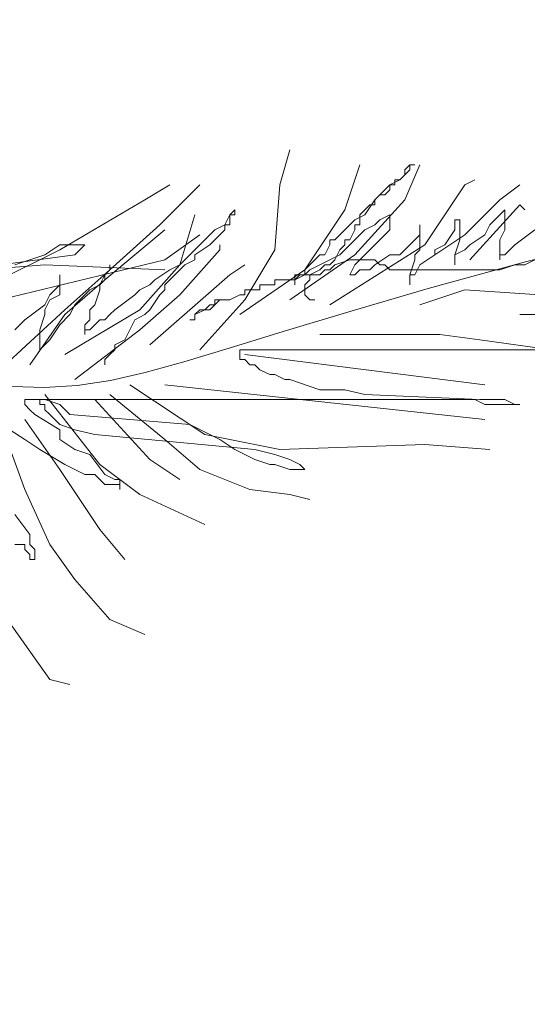
# Model space of a CAD drawing. Units: millimetres. Extents: x 595116 to 630915, y 909473 to 920225.
# Tile 85 of 134: x 629724.653 to 629727.558, y 919270.048 to 919275.684. Entities that reach past the tile are written whole.
import ezdxf

# ---------------------------------------------------------------- set-up
doc = ezdxf.new("R2010")
doc.units = ezdxf.units.MM
doc.layers.add('Dimension', color=3, linetype='Continuous', lineweight=18)
doc.layers.add('L-PLNT', color=85, linetype='Continuous', lineweight=13)
doc.styles.get("Standard").update_dxf_attribs({"font": 'arial.ttf'})
doc.dimstyles.new('ISO-25', dxfattribs={"dimtxt": 9, "dimasz": 6, "dimexe": 1.25, "dimexo": 0.625, "dimtad": 1, "dimlunit": 4, "dimtxsty": 'Standard', "dimcen": 2.5, "dimadec": 0, "dimazin": 0, "dimtfac": 1, "dimtmove": 0, "dimatfit": 3, "dimfxl": 1, "dimarcsym": 0})

# ---------------------------------------------------------------- blocks, each defined once
blk = doc.blocks.new('A$C4FB75ABC')
for p, q in [((4.2249, 2.058), (4.2402, 2.1114)), ((4.324, 2.0199), (4.3469, 2.0885)), ((4.4156, 2.0809), (4.4232, 2.0885)), ((4.4156, 2.0352), (4.4384, 2.0885)), ((4.4232, 2.0885), (4.4308, 2.0885)), ((4.4308, 2.0885), (4.4232, 2.0885)), ((4.4232, 2.0885), (4.4232, 2.0809)), ((4.4079, 2.0657), (4.4156, 2.0733)), ((4.4156, 2.0733), (4.4079, 2.0657)), ((4.4156, 2.0733), (4.4156, 2.0809)), ((4.4232, 2.0809), (4.4156, 2.0733)), ((4.019, 2.0352), (4.0571, 2.058)), ((4.0419, 1.9971), (4.1029, 2.058)), ((4.2173, 1.9589), (4.2249, 2.058)), ((4.3927, 2.058), (4.3851, 2.0504)), ((4.4079, 2.0657), (4.3927, 2.058)), ((4.3927, 2.0504), (4.3927, 2.058)), ((4.3927, 2.058), (4.4003, 2.058)), ((4.4003, 2.058), (4.4003, 2.0657)), ((4.4003, 2.0657), (4.4079, 2.0657)), ((4.4461, 1.9666), (4.5071, 2.058)), ((4.5071, 2.058), (4.5223, 2.0657)), ((4.5605, 2.0352), (4.591, 2.058)), ((4.3698, 2.0352), (4.3774, 2.0428)), ((4.3774, 2.0428), (4.3698, 2.0352)), ((4.3851, 2.0504), (4.3774, 2.0428)), ((4.3774, 2.0428), (4.3851, 2.0428)), ((4.3851, 2.0428), (4.3927, 2.0504)), ((3.8894, 1.9589), (4.019, 2.0352)), ((4.3393, 1.9513), (4.4156, 2.0352)), ((4.3469, 2.0123), (4.3622, 2.0275)), ((4.3698, 2.0352), (4.3546, 2.0123)), ((4.3622, 2.0275), (4.3698, 2.0275)), ((4.3698, 2.0275), (4.3698, 2.0352)), ((4.5071, 1.9818), (4.5605, 2.0352)), ((4.5147, 1.9437), (4.591, 2.0275)), ((4.591, 2.0275), (4.5986, 2.0199)), ((4.0724, 1.9361), (4.0953, 2.0123)), ((4.1486, 2.0123), (4.141, 1.9971)), ((4.1563, 2.0199), (4.1486, 2.0123)), ((4.1486, 1.9971), (4.1486, 2.0123)), ((4.1486, 2.0123), (4.1563, 2.0123)), ((4.1563, 2.0123), (4.1563, 2.0199)), ((4.263, 1.9285), (4.324, 2.0199)), ((4.3546, 2.0123), (4.3393, 2.0047)), ((4.3469, 1.9971), (4.3469, 2.0123)), ((4.3774, 2.0047), (4.3927, 2.0123)), ((4.3927, 2.0123), (4.3927, 1.9894)), ((4.5528, 2.0047), (4.5605, 2.0123)), ((4.5605, 2.0123), (4.5681, 2.0199)), ((4.5681, 2.0199), (4.5681, 1.9894)), ((4.3393, 2.0047), (4.3317, 1.9971)), ((4.3698, 1.9971), (4.3774, 2.0047)), ((4.4918, 1.9894), (4.4918, 2.0047)), ((4.4918, 2.0047), (4.4995, 2.0047)), ((4.4995, 2.0047), (4.4995, 1.9742)), ((4.5452, 1.9971), (4.5528, 2.0047)), ((3.958, 1.9132), (4.0495, 1.9894)), ((3.9656, 1.9285), (4.0419, 1.9971)), ((4.1258, 1.9894), (4.1181, 1.9818)), ((4.141, 1.9971), (4.1258, 1.9894)), ((4.1334, 1.9818), (4.141, 1.9894)), ((4.141, 1.9894), (4.141, 1.9971)), ((4.141, 1.9971), (4.1486, 1.9971)), ((4.3317, 1.9971), (4.3164, 1.9818)), ((4.3317, 1.9742), (4.3393, 1.9894)), ((4.3393, 1.9894), (4.3393, 1.9971)), ((4.3393, 1.9971), (4.3469, 1.9971)), ((4.3469, 1.9818), (4.3546, 1.9894)), ((4.3546, 1.9894), (4.3698, 1.9971)), ((4.3927, 1.9894), (4.3851, 1.9818)), ((4.4384, 1.9818), (4.4384, 1.9971)), ((4.4384, 1.9971), (4.4384, 1.9589)), ((4.4766, 1.9666), (4.4918, 1.9894)), ((4.5376, 1.9818), (4.5452, 1.9971)), ((4.5681, 1.9894), (4.5605, 1.9742)), ((4.5833, 1.9666), (4.6138, 1.9894)), ((4.7725, 1.9851), (4.5975, 1.9398)), ((4.0495, 1.9437), (4.1029, 1.9818)), ((4.1181, 1.9818), (4.1029, 1.9666)), ((4.1181, 1.9666), (4.1334, 1.9818)), ((4.3088, 1.9742), (4.3012, 1.9742)), ((4.3012, 1.9742), (4.3012, 1.9666)), ((4.3164, 1.9818), (4.3088, 1.9742)), ((4.3164, 1.9513), (4.3469, 1.9818)), ((4.324, 1.9666), (4.324, 1.9742)), ((4.324, 1.9742), (4.3317, 1.9742)), ((4.3851, 1.9818), (4.3698, 1.9666)), ((4.4156, 1.9589), (4.4308, 1.9742)), ((4.4308, 1.9742), (4.4384, 1.9818)), ((4.4384, 1.9361), (4.5071, 1.9818)), ((4.4995, 1.9742), (4.4918, 1.9513)), ((4.5147, 1.9666), (4.5376, 1.9818)), ((4.5605, 1.9742), (4.5605, 1.9437)), ((3.7521, 1.8903), (3.8894, 1.9589)), ((3.8894, 1.9666), (3.8665, 1.9513)), ((3.9275, 1.9666), (3.8894, 1.9666)), ((3.9122, 1.9513), (3.9199, 1.9589)), ((3.9199, 1.9589), (3.9275, 1.9666)), ((4.0724, 1.8903), (4.1334, 1.9589)), ((4.1029, 1.9666), (4.08, 1.9437)), ((4.0953, 1.9513), (4.1181, 1.9666)), ((4.1334, 1.9589), (4.1334, 1.9666)), ((4.1715, 1.8827), (4.2173, 1.9589)), ((4.3012, 1.9666), (4.2935, 1.9513)), ((4.3012, 1.8751), (4.4461, 1.9666)), ((4.3088, 1.9437), (4.3164, 1.9589)), ((4.3164, 1.9589), (4.324, 1.9666)), ((4.3622, 1.9589), (4.3469, 1.9437)), ((4.3698, 1.9666), (4.3622, 1.9589)), ((4.4079, 1.9513), (4.4156, 1.9589)), ((4.4384, 1.9589), (4.4308, 1.9513)), ((4.4613, 1.9589), (4.4766, 1.9666)), ((4.4613, 1.9513), (4.4613, 1.9589)), ((4.4918, 1.9513), (4.5071, 1.9589)), ((4.5071, 1.9589), (4.5147, 1.9666)), ((4.5681, 1.9513), (4.5757, 1.9589)), ((4.5757, 1.9589), (4.5833, 1.9666)), ((3.7445, 1.9285), (3.9122, 1.9513)), ((3.7978, 1.8827), (4.0495, 1.9437)), ((3.8665, 1.9513), (3.8207, 1.9361)), ((4.08, 1.9437), (4.0724, 1.9361)), ((4.08, 1.9361), (4.0953, 1.9437)), ((4.0953, 1.9437), (4.0953, 1.9513)), ((4.2402, 1.8827), (4.3393, 1.9513)), ((4.2859, 1.9513), (4.2707, 1.9361)), ((4.2707, 1.9285), (4.3012, 1.9437)), ((4.2935, 1.9513), (4.2859, 1.9513)), ((4.3012, 1.9437), (4.3164, 1.9513)), ((4.3012, 1.9361), (4.3088, 1.9437)), ((4.3317, 1.9437), (4.3088, 1.9361)), ((4.3698, 1.9437), (4.3317, 1.9437)), ((4.3469, 1.9437), (4.3393, 1.9361)), ((4.3698, 1.9361), (4.3927, 1.9513)), ((4.3774, 1.9361), (4.3698, 1.9437)), ((4.3927, 1.9513), (4.4079, 1.9513)), ((4.4308, 1.9437), (4.4232, 1.9208)), ((4.4308, 1.9513), (4.4308, 1.9437)), ((4.4384, 1.9361), (4.4613, 1.9513)), ((4.5975, 1.9398), (4.4513, 1.8996)), ((4.4918, 1.9513), (4.4918, 1.9361)), ((4.4918, 1.9361), (4.4918, 1.9513)), ((4.5605, 1.9513), (4.5681, 1.9513)), ((4.5605, 1.9437), (4.5605, 1.9513)), ((4.6138, 1.9437), (4.5986, 1.9361)), ((3.5843, 1.9132), (3.8665, 1.9361)), ((3.8665, 1.9361), (4.0495, 1.9285)), ((3.897, 1.8675), (3.9656, 1.9285)), ((3.958, 1.9208), (3.9656, 1.9285)), ((3.9656, 1.9285), (3.958, 1.9208)), ((3.9656, 1.9285), (3.9656, 1.9361)), ((3.9656, 1.9361), (3.9656, 1.9285)), ((4.0114, 1.8675), (4.0724, 1.9361)), ((4.0571, 1.9285), (4.0343, 1.9132)), ((4.0724, 1.9361), (4.0571, 1.9285)), ((4.0571, 1.9132), (4.0724, 1.9285)), ((4.0724, 1.9285), (4.08, 1.9361)), ((4.1486, 1.9208), (4.1715, 1.9361)), ((4.1639, 1.8599), (4.263, 1.9285)), ((4.2707, 1.9361), (4.263, 1.9285)), ((4.263, 1.9285), (4.263, 1.9208)), ((4.263, 1.9208), (4.2707, 1.9285)), ((4.2707, 1.9208), (4.2859, 1.9285)), ((4.2859, 1.9285), (4.2935, 1.9361)), ((4.2935, 1.9285), (4.2859, 1.9208)), ((4.2935, 1.9361), (4.3012, 1.9361)), ((4.3012, 1.9285), (4.2935, 1.9285)), ((4.3088, 1.9361), (4.3012, 1.9285)), ((4.3393, 1.9361), (4.3317, 1.9208)), ((4.3393, 1.9208), (4.3469, 1.9285)), ((4.3469, 1.9285), (4.3622, 1.9285)), ((4.3622, 1.9285), (4.3698, 1.9361)), ((4.3851, 1.9361), (4.3774, 1.9361)), ((4.3927, 1.9285), (4.3851, 1.9361)), ((4.5605, 1.9285), (4.3927, 1.9285)), ((4.4308, 1.9208), (4.4384, 1.9361)), ((4.5833, 1.9361), (4.5605, 1.9285)), ((4.5986, 1.9361), (4.5833, 1.9361)), ((3.8894, 1.8903), (3.8894, 1.9208)), ((3.8894, 1.9208), (3.8894, 1.9056)), ((3.897, 1.8599), (3.958, 1.9132)), ((3.958, 1.9208), (3.9504, 1.9056)), ((3.9504, 1.9056), (3.958, 1.9132)), ((3.958, 1.9132), (3.958, 1.9208)), ((4.0266, 1.8141), (4.1486, 1.9208)), ((4.0343, 1.9132), (4.0266, 1.9056)), ((4.0495, 1.9056), (4.0571, 1.9132)), ((4.2478, 1.9132), (4.2173, 1.9132)), ((4.2173, 1.9132), (4.2173, 1.9056)), ((4.2554, 1.9208), (4.2478, 1.9132)), ((4.2478, 1.9056), (4.2478, 1.9208)), ((4.2478, 1.9208), (4.263, 1.9208)), ((4.263, 1.9208), (4.2478, 1.9132)), ((4.2478, 1.9132), (4.2478, 1.9056)), ((4.263, 1.9208), (4.2554, 1.9208)), ((4.2859, 1.9208), (4.263, 1.9208)), ((4.263, 1.9056), (4.2707, 1.9132)), ((4.2707, 1.9132), (4.2707, 1.9208)), ((4.3317, 1.9208), (4.3393, 1.9208)), ((4.4232, 1.9208), (4.4232, 1.9056)), ((4.4232, 1.9056), (4.4232, 1.9208)), ((4.4232, 1.9208), (4.4308, 1.9208)), ((3.8894, 1.9056), (3.8741, 1.8903)), ((3.9351, 1.898), (3.9122, 1.8751)), ((3.9504, 1.9056), (3.9351, 1.898)), ((3.9427, 1.8751), (3.9504, 1.898)), ((3.9504, 1.898), (3.9504, 1.9056)), ((4.0114, 1.898), (4.0037, 1.8903)), ((4.0266, 1.9056), (4.0114, 1.898)), ((4.0419, 1.8903), (4.0495, 1.898)), ((4.0495, 1.898), (4.0495, 1.9056)), ((4.1944, 1.898), (4.1715, 1.898)), ((4.1715, 1.898), (4.1715, 1.8903)), ((4.2173, 1.9056), (4.1944, 1.9056)), ((4.1944, 1.9056), (4.1944, 1.898)), ((4.263, 1.8903), (4.263, 1.9056)), ((4.4513, 1.8996), (4.3302, 1.8644)), ((4.4384, 1.8751), (4.5071, 1.898)), ((4.5071, 1.898), (4.6215, 1.8903)), ((3.8741, 1.8903), (3.8665, 1.8751)), ((3.8665, 1.8675), (3.8741, 1.8827)), ((3.8741, 1.8827), (3.8894, 1.8903)), ((4.0037, 1.8903), (3.9732, 1.8675)), ((4.0114, 1.837), (4.0724, 1.8903)), ((4.0266, 1.8675), (4.0419, 1.8903)), ((4.1029, 1.8065), (4.1715, 1.8827)), ((4.1334, 1.8827), (4.1258, 1.8751)), ((4.1258, 1.8751), (4.1258, 1.8827)), ((4.1258, 1.8827), (4.1334, 1.8827)), ((4.1486, 1.8827), (4.1334, 1.8827)), ((4.1639, 1.8903), (4.1486, 1.8827)), ((4.1715, 1.8903), (4.1639, 1.8903)), ((4.2707, 1.8827), (4.263, 1.8903)), ((4.2783, 1.8827), (4.2707, 1.8827)), ((3.7978, 1.776), (3.897, 1.8675)), ((3.8665, 1.8751), (3.836, 1.8522)), ((3.8665, 1.8599), (3.8665, 1.8675)), ((3.897, 1.7989), (4.0114, 1.8675)), ((3.9122, 1.8751), (3.9046, 1.8599)), ((3.9351, 1.8675), (3.9427, 1.8751)), ((3.9351, 1.8522), (3.9351, 1.8675)), ((3.9732, 1.8675), (3.9656, 1.8599)), ((4.019, 1.8599), (4.0266, 1.8675)), ((4.1029, 1.8675), (4.0953, 1.8599)), ((4.0953, 1.8599), (4.1105, 1.8675)), ((4.1105, 1.8675), (4.1029, 1.8675)), ((4.1181, 1.8751), (4.1105, 1.8675)), ((4.1105, 1.8675), (4.1181, 1.8675)), ((4.1258, 1.8751), (4.1181, 1.8751)), ((4.1181, 1.8675), (4.1258, 1.8751)), ((4.3302, 1.8644), (4.2303, 1.8341)), ((3.836, 1.8522), (3.8207, 1.837)), ((3.8436, 1.7836), (3.897, 1.8599)), ((3.8589, 1.837), (3.8665, 1.8599)), ((3.9046, 1.8599), (3.8894, 1.8446)), ((3.9275, 1.8446), (3.9351, 1.8522)), ((3.9504, 1.8522), (3.9427, 1.8446)), ((3.958, 1.8522), (3.9504, 1.8522)), ((3.9656, 1.8599), (3.958, 1.8522)), ((3.9885, 1.8217), (4.0037, 1.8522)), ((4.0037, 1.8522), (4.019, 1.8599)), ((4.0953, 1.8522), (4.0876, 1.8522)), ((4.0876, 1.8522), (4.0953, 1.8522)), ((4.0953, 1.8599), (4.0953, 1.8522)), ((4.0953, 1.8522), (4.0953, 1.8599)), ((4.6062, 1.8599), (4.591, 1.8599)), ((4.591, 1.8599), (4.652, 1.8599)), ((3.8589, 1.8065), (3.8589, 1.837)), ((3.8894, 1.8446), (3.8741, 1.8217)), ((3.9122, 1.7608), (4.0114, 1.837)), ((3.9275, 1.8294), (3.9275, 1.8446)), ((3.9351, 1.837), (3.9275, 1.837)), ((3.9275, 1.837), (3.9275, 1.8294)), ((3.9427, 1.8446), (3.9351, 1.837)), ((4.2303, 1.8341), (4.1477, 1.8087)), ((3.8741, 1.8217), (3.8665, 1.8141)), ((3.9732, 1.8141), (3.9885, 1.8217)), ((4.2859, 1.8294), (4.4689, 1.8294)), ((4.4689, 1.8294), (4.53, 1.8217)), ((4.53, 1.8217), (4.6367, 1.8065)), ((3.8665, 1.8141), (3.8589, 1.8065)), ((3.9656, 1.7989), (3.9732, 1.8065)), ((3.9732, 1.8065), (3.9732, 1.8141)), ((4.1477, 1.8087), (4.0788, 1.7878)), ((4.1639, 1.7913), (4.1639, 1.8065)), ((4.1639, 1.8065), (5.0333, 1.8065)), ((3.958, 1.7913), (3.9656, 1.7989)), ((3.958, 1.7836), (3.958, 1.7913)), ((4.0788, 1.7878), (4.0197, 1.7715)), ((4.1715, 1.7913), (4.1639, 1.7913)), ((4.1715, 1.7989), (4.5376, 1.7531)), ((4.1792, 1.7836), (4.1715, 1.7913)), ((4.1868, 1.7836), (4.1792, 1.7836)), ((4.1944, 1.776), (4.1868, 1.7836)), ((4.2097, 1.7684), (4.1944, 1.776)), ((3.9666, 1.7597), (3.916, 1.7521)), ((4.0197, 1.7715), (3.9666, 1.7597)), ((4.2173, 1.7684), (4.2097, 1.7684)), ((4.2325, 1.7608), (4.2173, 1.7684)), ((4.2402, 1.7608), (4.2325, 1.7608)), ((4.2859, 1.7455), (4.2402, 1.7608)), ((3.8664, 1.749), (3.8165, 1.7504)), ((3.916, 1.7521), (3.8664, 1.749)), ((3.9961, 1.7531), (4.1105, 1.6769)), ((4.0495, 1.7531), (4.5376, 1.6998)), ((4.324, 1.7455), (4.2859, 1.7455)), ((4.3546, 1.7379), (4.324, 1.7455)), ((3.836, 1.7227), (3.836, 1.7303)), ((3.836, 1.7303), (3.8665, 1.7303)), ((3.8589, 1.7227), (3.8589, 1.7303)), ((3.8589, 1.7303), (4.5223, 1.7303)), ((3.8665, 1.7379), (3.9504, 1.6312)), ((3.8665, 1.7303), (3.8894, 1.7227)), ((3.9427, 1.7303), (4.0266, 1.6388)), ((3.9656, 1.7379), (4.0495, 1.6693)), ((4.53, 1.7303), (4.3546, 1.7379)), ((4.5223, 1.7303), (4.5376, 1.7227)), ((4.5681, 1.7303), (4.53, 1.7303)), ((4.5833, 1.7227), (4.5681, 1.7303)), ((3.8436, 1.715), (3.836, 1.7227)), ((3.8512, 1.7074), (3.8436, 1.715)), ((3.8665, 1.7227), (3.8589, 1.7227)), ((3.8665, 1.715), (3.8665, 1.7227)), ((3.8741, 1.7074), (3.8665, 1.715)), ((3.8894, 1.7227), (3.9046, 1.7074)), ((4.5376, 1.7227), (4.591, 1.7227)), ((4.591, 1.7227), (4.5833, 1.7227)), ((3.836, 1.6998), (3.8894, 1.6236)), ((3.8894, 1.6845), (3.8512, 1.7074)), ((3.8894, 1.6922), (3.8741, 1.7074)), ((3.9046, 1.7074), (4.0876, 1.6922)), ((3.8131, 1.6845), (3.836, 1.6693)), ((3.9122, 1.6845), (3.8894, 1.6922)), ((3.8894, 1.6693), (3.8894, 1.6845)), ((3.9427, 1.6769), (3.9122, 1.6845)), ((4.0876, 1.6922), (4.1181, 1.6769)), ((3.8055, 1.6769), (3.836, 1.5931)), ((3.836, 1.6693), (3.8589, 1.6541)), ((3.9122, 1.6541), (3.8894, 1.6693)), ((4.1868, 1.6541), (3.9427, 1.6769)), ((4.0495, 1.6693), (4.1029, 1.6236)), ((4.1105, 1.6769), (4.2249, 1.6541)), ((4.1181, 1.6769), (4.1334, 1.6693)), ((4.1334, 1.6693), (4.1563, 1.6541)), ((3.8589, 1.6541), (3.897, 1.6312)), ((3.9351, 1.6464), (3.9122, 1.6541)), ((4.1563, 1.6541), (4.1868, 1.6388)), ((4.2173, 1.6464), (4.1868, 1.6541)), ((4.2249, 1.6541), (4.4461, 1.6617)), ((4.4461, 1.6617), (4.5452, 1.6541)), ((3.958, 1.6159), (3.9351, 1.6464)), ((4.0266, 1.6388), (4.0724, 1.6083)), ((4.1868, 1.6388), (4.2097, 1.6312)), ((4.2402, 1.6388), (4.2173, 1.6464)), ((4.2554, 1.6312), (4.2402, 1.6388)), ((3.8894, 1.6236), (3.9504, 1.5321)), ((3.897, 1.6312), (3.9275, 1.6159)), ((3.9504, 1.6312), (4.0114, 1.5855)), ((4.1029, 1.6236), (4.1792, 1.5931)), ((4.2097, 1.6312), (4.2173, 1.6312)), ((4.2173, 1.6312), (4.2402, 1.6236)), ((4.2402, 1.6236), (4.263, 1.6236)), ((4.263, 1.6236), (4.2554, 1.6312)), ((3.9275, 1.6159), (3.9427, 1.6159)), ((3.9427, 1.6159), (3.958, 1.6007)), ((3.9732, 1.6083), (3.958, 1.6159)), ((3.9809, 1.6083), (3.9732, 1.6083)), ((3.9809, 1.5931), (3.9809, 1.6083)), ((3.836, 1.5931), (3.8741, 1.5092)), ((3.958, 1.6007), (3.9809, 1.6007)), ((3.9809, 1.6007), (3.9809, 1.5931)), ((4.1792, 1.5931), (4.2402, 1.5855)), ((4.0114, 1.5855), (4.1105, 1.5397)), ((4.2402, 1.5855), (4.2707, 1.5778)), ((3.8436, 1.5245), (3.8207, 1.555)), ((3.9504, 1.5321), (3.9885, 1.4864)), ((3.8436, 1.5092), (3.8436, 1.5245)), ((3.8207, 1.5092), (3.836, 1.5092)), ((3.836, 1.5092), (3.836, 1.5016)), ((3.8512, 1.5016), (3.8436, 1.5092)), ((3.8741, 1.5092), (3.9122, 1.4559)), ((3.836, 1.5016), (3.8436, 1.494)), ((3.8436, 1.494), (3.8436, 1.4864)), ((3.8512, 1.4864), (3.8512, 1.5016)), ((3.8436, 1.4864), (3.8512, 1.4864)), ((3.9122, 1.4559), (3.9656, 1.3949)), ((3.7826, 1.433), (3.8741, 1.3034)), ((3.9656, 1.3949), (4.019, 1.372)), ((3.8741, 1.3034), (3.9046, 1.2958))]:
    blk.add_line(p, q)
blk = doc.blocks.new('*D216')
at = {"layer": 'Defpoints', "color": 0, "transparency": 16777216}
for p in [(629743.5408, 919411.9276), (629505.0408, 919411.8279), (629743.5408, 918832.3776)]:
    blk.add_point(p, dxfattribs=at)
at = {"layer": 'Dimension', "color": 0, "lineweight": -2, "transparency": 16777216}
for p, q in [((629743.5408, 919411.3026), (629743.5408, 918831.1276)), ((629505.0408, 919411.2029), (629505.0408, 918831.1276)), ((629511.0408, 918832.3776), (629737.5408, 918832.3776))]:
    blk.add_line(p, q, dxfattribs=at)
at = {"layer": 'Dimension', "color": 0, "transparency": 16777216}
for points in [[(629511.0408, 918833.3776), (629511.0408, 918831.3776), (629505.0408, 918832.3776)], [(629737.5408, 918833.3776), (629737.5408, 918831.3776), (629743.5408, 918832.3776)]]:
    blk.add_solid(points, dxfattribs=at)
at = {"layer": 'Dimension', "color": 0, "transparency": 16777216, "insert": (629624.2908, 918837.656), "char_height": 9, "attachment_point": 5}
blk.add_mtext('19\'-10 1/2"', dxfattribs=at)

msp = doc.modelspace()

# ---------------------------------------------------------------- block references
at = {"layer": 'L-PLNT', "xscale": 3.753413438031968, "yscale": 3.753413438031968, "zscale": 3.753413438031968}
msp.add_blockref('A$C4FB75ABC', (629710.2837, 919267.0144), dxfattribs=at)

# ---------------------------------------------------------------- dimensions: what is measured, and where the dimension line sits
at = {"layer": 'Dimension'}
dim = msp.add_linear_dim(base=(629743.5408, 918832.3776), p1=(629505.0408, 919411.8279), p2=(629743.5408, 919411.9276), dimstyle='ISO-25', override={"dimdec": 1, "dimlfac": 1, "dimrnd": 0, "dimzin": 1, "dimdsep": 46, "dimlunit": 4, "dimfrac": 2}, dxfattribs=at)
dim.commit()
dim.dimension.update_dxf_attribs({"geometry": '*D216', "text_midpoint": (629624.2908, 918837.656)})

doc.saveas('drawing.dxf')
